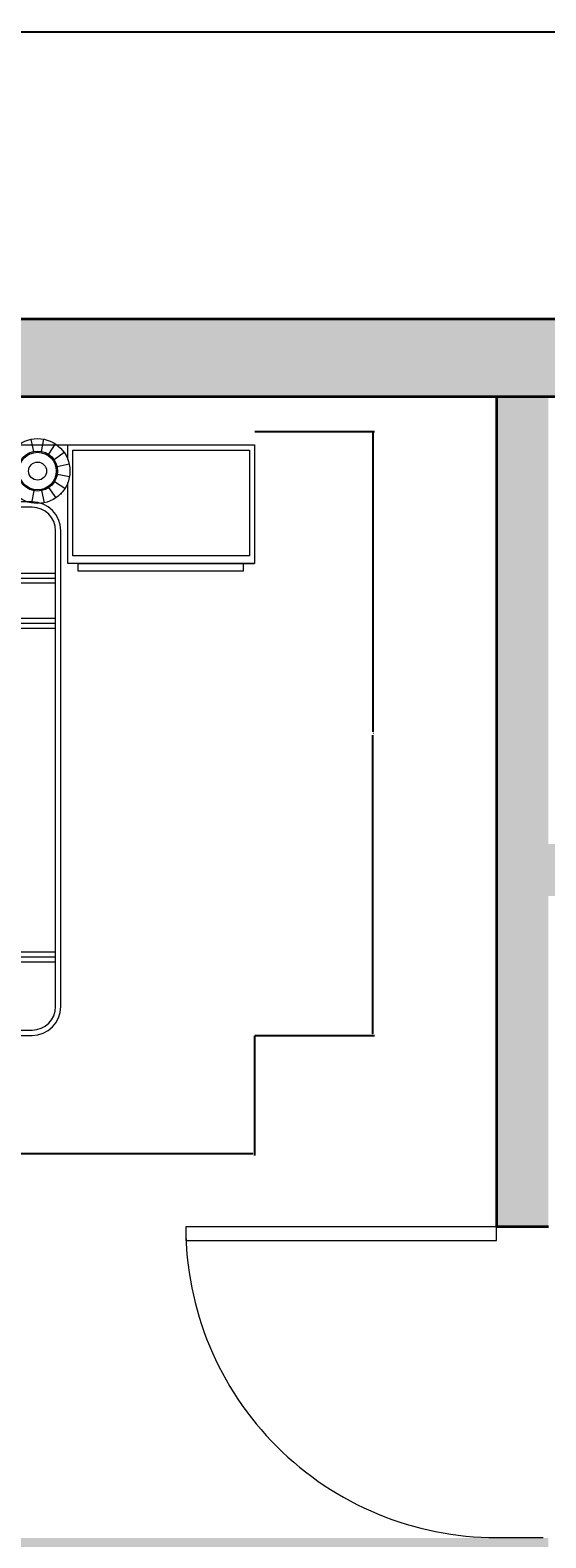
# Model space of a CAD drawing. Units: inches. Extents: x 2070 to 4408, y 1595 to 4269.
# Tile 14 of 20: x 2185 to 2245, y 2150 to 2325. Entities that reach past the tile are written whole.
import ezdxf

# ---------------------------------------------------------------- set-up
doc = ezdxf.new("R2010")
doc.units = ezdxf.units.IN
for name, color, linetype, lineweight in [('A-ANNO-DIMS', 2, 'Continuous', 18), ('A-DOOR', 4, 'Continuous', 18), ('A-FURN', 8, 'Continuous', 18), ('A-WALL', 7, 'Continuous', 35)]:
    doc.layers.add(name, color=color, linetype=linetype, lineweight=lineweight)
doc.layers.add('A-WALL-PATT', color=18, linetype='Continuous', lineweight=13, true_color=0x000000)
doc.styles.get("Standard").update_dxf_attribs({"font": 'arial.ttf'})
doc.dimstyles.get("Standard").update_dxf_attribs({"dimtxt": 0.18, "dimasz": 0.18, "dimexe": 0.18, "dimexo": 0.0625, "dimgap": 0.09, "dimtad": 0, "dimtih": 1, "dimtoh": 1, "dimdec": 4, "dimzin": 0, "dimdsep": 46, "dimtxsty": 'Standard', "dimcen": 0.09, "dimadec": 0, "dimazin": 0, "dimtfac": 1, "dimtdec": 4, "dimtofl": 0, "dimtmove": 0, "dimatfit": 3, "dimfxl": 1, "dimtolj": 1, "dimtzin": 0, "dimarcsym": 0})

# ---------------------------------------------------------------- blocks, each defined once
blk = doc.blocks.new('*U3')
for p, q in [((0, 0), (0, 6)), ((40, 0), (40, 6))]:
    blk.add_line(p, q)
blk.add_lwpolyline([(0, 0), (0, -40), (1.75, -40), (1.75, 0)], close=True)
blk.add_arc((0, 0), 40, 270, 0)
blk = doc.blocks.new('A$C18EB7ED0')
for p, q in [((0, 2.1539), (2.8801, 2.1539)), ((2.0643, 2.1733), (2.0739, 2.129)), ((2.1105, 2.1741), (2.1024, 2.1295)), ((2.1534, 2.1571), (2.1288, 2.119)), ((2.1997, 2.1), (2.1997, 2.1539)), ((2.8801, 2.1539), (2.8801, 1.7209)), ((2.1865, 2.1251), (2.1493, 2.0992)), ((2.2184, 2.1337), (2.8624, 2.1337)), ((2.2184, 1.7489), (2.2184, 2.1337)), ((2.8624, 2.1337), (2.8624, 1.7489)), ((2.2049, 2.0827), (2.1606, 2.0731)), ((2.2056, 2.0366), (2.161, 2.0447)), ((2.0682, 1.9414), (2.0763, 1.986)), ((2.1143, 1.9422), (2.1047, 1.9865)), ((2.1566, 1.9605), (2.1308, 1.9978)), ((2.1887, 1.9937), (2.1506, 2.0183)), ((2.1997, 1.7209), (2.1997, 2.0155)), ((2.0691, 1.9452), (0.8491, 1.9452)), ((2.0691, 1.926), (0.8491, 1.926)), ((2.1742, 1.9754), (2.1771, 1.9754)), ((2.1771, 1.9754), (2.1771, 1.9785)), ((2.155, 0.1052), (2.155, 1.8401)), ((2.1743, 0.1052), (2.1743, 1.8401)), ((2.8801, 1.7209), (2.1997, 1.7209)), ((2.8624, 1.7489), (2.2184, 1.7489)), ((2.2369, 1.7209), (2.8801, 1.7209)), ((2.2369, 1.6929), (2.2369, 1.7209)), ((2.839, 1.7209), (2.839, 1.6929)), ((1.9608, 1.6858), (2.155, 1.6858)), ((1.9608, 1.6678), (2.155, 1.6678)), ((1.9608, 1.6498), (2.155, 1.6498)), ((2.839, 1.6929), (2.2369, 1.6929)), ((0.7632, 1.5215), (2.155, 1.5215)), ((0.7632, 1.5035), (2.155, 1.5035)), ((0.7632, 1.4855), (2.155, 1.4855)), ((0.7632, 0.3045), (2.155, 0.3045)), ((0.7632, 0.2865), (2.155, 0.2865)), ((0.7632, 0.2685), (2.155, 0.2685)), ((0.8491, 0.0193), (2.0691, 0.0193)), ((0.8491, 0), (2.0691, 0))]:
    blk.add_line(p, q)
for radius in [0.1182, 0.0729, 0.0684, 0.0328]:
    blk.add_circle((2.0893, 2.0578), radius)
for centre, radius, start, end in [((2.0691, 1.8401), 0.1052, 0, 90), ((2.0691, 1.8401), 0.0859, 0, 90), ((2.0691, 0.1052), 0.1052, 270, 0), ((2.0691, 0.1052), 0.0859, 270, 0)]:
    blk.add_arc(centre, radius, start, end)
blk = doc.blocks.new('*D17')
at = {"layer": 'A-ANNO-DIMS', "color": 0, "lineweight": -2, "transparency": 16777216}
for p, q in [((2119.88, 2208.47), (2119.88, 2194.65)), ((2211.2, 2208.47), (2211.2, 2194.65)), ((2120.06, 2194.83), (2164.77, 2194.83)), ((2211.02, 2194.83), (2166.31, 2194.83))]:
    blk.add_line(p, q, dxfattribs=at)
at = {"layer": 'A-ANNO-DIMS', "color": 0, "transparency": 16777216}
for points in [[(2120.06, 2194.86), (2120.06, 2194.8), (2119.88, 2194.83)], [(2211.02, 2194.86), (2211.02, 2194.8), (2211.2, 2194.83)]]:
    blk.add_solid(points, dxfattribs=at)
at = {"layer": 'Defpoints', "color": 0, "transparency": 16777216}
for p in [(2119.88, 2208.53), (2211.2, 2208.53), (2211.2, 2194.83)]:
    blk.add_point(p, dxfattribs=at)
at = {"layer": 'A-ANNO-DIMS', "color": 0, "transparency": 16777216, "insert": (2165.54, 2194.83), "char_height": 0.18, "attachment_point": 5}
blk.add_mtext('\\A1;BED SET 91', dxfattribs=at)
blk = doc.blocks.new('*D18')
at = {"layer": 'A-ANNO-DIMS', "color": 0, "lineweight": -2, "transparency": 16777216}
for p, q in [((2211.26, 2278.36), (2225.08, 2278.36)), ((2224.9, 2278.18), (2224.9, 2243.63)), ((2224.9, 2208.71), (2224.9, 2243.26)), ((2211.26, 2208.53), (2225.08, 2208.53))]:
    blk.add_line(p, q, dxfattribs=at)
at = {"layer": 'A-ANNO-DIMS', "color": 0, "transparency": 16777216}
for points in [[(2224.87, 2278.18), (2224.93, 2278.18), (2224.9, 2278.36)], [(2224.87, 2208.71), (2224.93, 2208.71), (2224.9, 2208.53)]]:
    blk.add_solid(points, dxfattribs=at)
at = {"layer": 'Defpoints', "color": 0, "transparency": 16777216}
for p in [(2211.2, 2278.36), (2224.9, 2278.36), (2211.2, 2208.53)]:
    blk.add_point(p, dxfattribs=at)
at = {"layer": 'A-ANNO-DIMS', "color": 0, "transparency": 16777216, "insert": (2224.9, 2243.45), "char_height": 0.18, "attachment_point": 5}
blk.add_mtext('\\A1;70', dxfattribs=at)
blk = doc.blocks.new('*D23')
at = {"layer": 'A-ANNO-DIMS', "color": 0, "lineweight": -2, "transparency": 16777216}
for p, q in [((2103.2, 2291.46), (2103.2, 2324.76)), ((2103.38, 2324.58), (2278.91, 2324.58)), ((2455.02, 2324.58), (2279.48, 2324.58)), ((2455.2, 2291.46), (2455.2, 2324.76))]:
    blk.add_line(p, q, dxfattribs=at)
at = {"layer": 'A-ANNO-DIMS', "color": 0, "transparency": 16777216}
for points in [[(2103.38, 2324.61), (2103.38, 2324.55), (2103.2, 2324.58)], [(2455.02, 2324.61), (2455.02, 2324.55), (2455.2, 2324.58)]]:
    blk.add_solid(points, dxfattribs=at)
at = {"layer": 'Defpoints', "color": 0, "transparency": 16777216}
for p in [(2455.2, 2324.58), (2103.2, 2291.4), (2455.2, 2291.4)]:
    blk.add_point(p, dxfattribs=at)
at = {"layer": 'A-ANNO-DIMS', "color": 0, "transparency": 16777216, "insert": (2279.2, 2324.58), "char_height": 0.18, "attachment_point": 5}
blk.add_mtext('\\A1;352', dxfattribs=at)
blk = doc.blocks.new('*D24')
at = {"layer": 'A-ANNO-DIMS', "color": 0, "lineweight": -2, "transparency": 16777216}
for p, q in [((2103.13, 2291.4), (2069.84, 2291.4)), ((2070.02, 2291.22), (2070.02, 1960.08)), ((2070.02, 1628.58), (2070.02, 1959.72)), ((2336.13, 1628.4), (2069.84, 1628.4))]:
    blk.add_line(p, q, dxfattribs=at)
at = {"layer": 'A-ANNO-DIMS', "color": 0, "transparency": 16777216}
for points in [[(2069.99, 2291.22), (2070.05, 2291.22), (2070.02, 2291.4)], [(2069.99, 1628.58), (2070.05, 1628.58), (2070.02, 1628.4)]]:
    blk.add_solid(points, dxfattribs=at)
at = {"layer": 'Defpoints', "color": 0, "transparency": 16777216}
for p in [(2070.02, 2291.4), (2103.2, 2291.4), (2336.2, 1628.4)]:
    blk.add_point(p, dxfattribs=at)
at = {"layer": 'A-ANNO-DIMS', "color": 0, "transparency": 16777216, "insert": (2070.02, 1959.9), "char_height": 0.18, "attachment_point": 5}
blk.add_mtext('\\A1;663', dxfattribs=at)

msp = doc.modelspace()

# ---------------------------------------------------------------- hatches: boundary and pattern name
at = {"layer": 'A-WALL-PATT'}
h = msp.add_hatch(color=256, dxfattribs=at)
h.dxf.hatch_style = 1
h.paths.add_polyline_path([(2346.196, 2218.3995), (2346.196, 2282.3995), (2340.196, 2282.3995), (2340.196, 2212.3995), (2345.5866, 2212.3995), (2346.196, 2212.3995)], flags=0)
h.paths.add_polyline_path([(2245.196, 2282.3995), (2239.196, 2282.3995), (2239.196, 2186.3995), (2244.5866, 2186.3995), (2245.196, 2186.3995)], flags=0)
h.paths.add_polyline_path([(2340.196, 2230.6455), (2245.196, 2230.6455), (2245.196, 2224.6455), (2340.196, 2224.6455)], flags=0)
h.paths.add_polyline_path([(2245.196, 2150.3995), (2239.196, 2150.3995), (2164.4362, 2150.3995), (2164.4362, 2144.3995), (2239.196, 2144.3995), (2239.196, 2086.3995), (2239.196, 2067.2711), (2244.5866, 2067.2711), (2245.196, 2067.2711), (2245.196, 2144.3995)], flags=0)
h.paths.add_polyline_path([(2346.196, 2176.3995), (2340.196, 2176.3995), (2340.196, 2086.3995), (2346.196, 2086.3995), (2346.196, 2125.318)], flags=0)
h.paths.add_polyline_path([(2446.196, 2086.3995), (2346.196, 2086.3995), (2340.196, 2086.3995), (2340.196, 2080.3995), (2446.196, 2080.3995)], flags=0)
h.paths.add_polyline_path([(2455.196, 2291.3995), (2103.196, 2291.3995), (2103.196, 1699.3995), (2336.196, 1699.3995), (2336.196, 1628.3995), (2345.196, 1628.3995), (2446.196, 1628.3995), (2454.8846, 1628.3995), (2454.8846, 1699.3995)])
h.paths.add_polyline_path([(2446.196, 2282.3995), (2446.196, 2218.3995), (2446.196, 2212.3995), (2446.196, 2086.3995), (2446.196, 2080.3995), (2446.196, 1708.3995), (2446.196, 1637.3995), (2345.196, 1637.3995), (2345.196, 1699.3995), (2345.196, 1708.3995), (2336.196, 1708.3995), (2112.196, 1708.3995), (2112.196, 2282.3995), (2239.196, 2282.3995), (2245.196, 2282.3995), (2356.196, 2282.3995)], flags=16)
h.paths.add_polyline_path([(2245.196, 2150.3995), (2245.196, 2144.3995), (2245.196, 2067.2711), (2244.5866, 2067.2711), (2239.196, 2067.2711), (2239.196, 2065.6988), (2203.2929, 2065.6988, 0.40145271), (2239.196, 2031.3337), (2244.5866, 2031.3337), (2245.196, 2031.2711), (2245.196, 1924.1525), (2239.196, 1924.1525), (2239.196, 1922.5803), (2203.2929, 1922.5803, 0.40145271), (2239.196, 1888.2151), (2244.5866, 1888.2151), (2245.196, 1888.1525), (2245.196, 1748.3995), (2339.196, 1748.4621, -0.40145271), (2303.2929, 1782.8272), (2303.2585, 1782.8272), (2303.2585, 1784.3995), (2339.196, 1784.3995), (2339.196, 1877.2067), (2291.196, 1877.2067), (2291.196, 1883.2067), (2291.196, 1946.3995), (2291.196, 1952.3995), (2291.196, 2086.3995), (2297.196, 2086.3995), (2302.196, 2086.3995), (2302.196, 2081.0259), (2303.7633, 2081.0259), (2303.7633, 2080.3995), (2338.0148, 2080.3995, 0.00437129), (2338.0203, 2081.0259), (2338.0203, 2086.3995), (2340.196, 2086.3995), (2340.196, 2176.4621), (2345.5866, 2176.4621, 0.40145271), (2381.4896, 2210.8272), (2345.5866, 2210.8272), (2345.5866, 2212.3995), (2340.196, 2212.3995), (2340.196, 2224.6455), (2245.196, 2224.6455), (2245.196, 2186.3995), (2244.5866, 2186.3995), (2239.196, 2186.3995), (2239.196, 2184.8272), (2203.2929, 2184.8272, 0.40145271), (2239.196, 2150.4621), (2244.5866, 2150.4621)], flags=0)
h.paths.add_polyline_path([(2346.196, 2282.3995), (2346.196, 2218.3995), (2377.1813, 2218.3995), (2377.1813, 2212.3995), (2346.196, 2212.3995), (2345.5866, 2212.3995), (2340.196, 2212.3995), (2340.196, 2224.6455), (2245.196, 2224.6455), (2245.196, 2230.6455), (2245.196, 2282.3995), (2292.696, 2256.5225), (2340.196, 2282.3995)], flags=0)
h.paths.add_polyline_path([(2346.196, 2086.3995), (2340.196, 2086.3995), (2340.196, 2080.3995), (2446.196, 2080.3995), (2431.196, 2016.3995), (2446.196, 1952.3995), (2412.196, 1952.3995), (2412.196, 2080.3995), (2340.196, 2080.3995), (2340.196, 2086.3995), (2340.196, 2176.3995), (2346.196, 2176.3995), (2346.196, 2125.318)], flags=0)
h.paths.add_polyline_path([(2186.508, 2270.0471, -0.03755288), (2186.9712, 2269.8581), (2186.9164, 2270.112, -0.02759121)], flags=0)
h.paths.add_polyline_path([(2183.955, 2273.7766, 1), (2188.2945, 2273.7766, 1)], flags=0)
h.paths.add_polyline_path([(2142.5261, 2274.6158, -0.03707541), (2142.5672, 2275.1696), (2142.5672, 2276.826), (2119.8759, 2276.826), (2119.8759, 2263.0962), (2140.4332, 2263.0962), (2142.5672, 2263.0962), (2142.5672, 2274.0621, -0.03707541)], flags=0)
h.paths.add_polyline_path([(2209.8974, 2263.0962), (2209.8974, 2262.2079), (2190.8042, 2262.2079), (2190.8042, 2263.0962)], flags=0)
h.paths.add_polyline_path([(2210.6382, 2276.1833), (2210.6382, 2263.9844), (2190.2185, 2263.9844), (2190.2185, 2276.1833)], flags=0)
h.paths.add_polyline_path([(2188.4362, 2273.7766, -1), (2183.8133, 2273.7766, -1)], flags=0)
h.paths.add_polyline_path([(2245.196, 2150.3995), (2245.196, 2144.3995), (2245.196, 2067.2711), (2239.196, 2067.2711), (2239.196, 2080.3995), (2172.196, 2080.3995), (2172.196, 2000.3995), (2239.196, 2000.3995), (2239.196, 1940.3995), (2159.0187, 1940.3995), (2123.0187, 1940.3995), (2112.196, 1940.3995), (2112.196, 1946.3995), (2123.0187, 1946.3995), (2123.0187, 1982.2238), (2124.586, 1982.2238), (2124.586, 1982.1895, -0.40145271), (2158.8429, 1946.3995), (2159.0187, 1946.3995), (2239.196, 1946.3995), (2239.196, 1994.3995), (2112.196, 1994.3995), (2112.196, 2000.3995), (2139.196, 2040.3995), (2112.196, 2080.3995), (2112.196, 2086.3995), (2239.196, 2086.3995), (2239.196, 2144.3995), (2209.5809, 2144.3995), (2209.5809, 2136.3995), (2203.0809, 2136.3995), (2205.0809, 2130.3996, -0.70257121), (2199.081, 2116.3995, -0.70256205), (2193.0809, 2130.3994), (2195.0809, 2136.3995), (2192.0809, 2136.3995), (2192.0809, 2134.8995), (2189.0809, 2134.8995), (2189.0809, 2135.8995), (2191.0809, 2135.8995), (2191.0809, 2136.3995), (2188.5809, 2136.3995), (2188.5809, 2144.3995), (2164.2481, 2144.3995, -0.39385849), (2130.0035, 2109.5491), (2130.0035, 2109.5147), (2128.4362, 2109.5147), (2128.4362, 2144.3995), (2112.196, 2144.3995), (2112.196, 2150.3995), (2128.4362, 2150.3995), (2128.4362, 2150.7127), (2164.4362, 2150.7127), (2164.4362, 2150.3995), (2239.196, 2150.3995)], flags=0)
h.paths.add_polyline_path([(2188.2075, 2266.8735), (2188.2075, 2211.8632, -0.41421356), (2185.4833, 2209.1391), (2146.7995, 2209.1391, -0.41421356), (2144.0754, 2211.8632), (2144.0754, 2266.8735, -0.41421356), (2146.7995, 2269.5976), (2185.4833, 2269.5976, -0.41421356)], flags=0)
h.paths.add_polyline_path([(2185.0844, 2273.7766, -1), (2187.1651, 2273.7766, -1)], flags=0)
h.paths.add_polyline_path([(2182.0486, 2259.2932), (2168.0953, 2259.2932), (2168.0953, 2260.8424), (2163.7261, 2260.8424), (2163.7261, 2259.2932), (2149.7727, 2259.2932), (2149.7727, 2266.3352), (2163.7261, 2266.3352), (2163.7261, 2261.9839), (2168.0953, 2261.9839), (2168.0953, 2266.3352), (2182.0486, 2266.3352)], flags=0)
h.paths.add_polyline_path([(2148.2585, 2250.2051), (2153.0615, 2241.8861, 0.39807048)], flags=0)
h.paths.add_polyline_path([(2162.7572, 2247.2885), (2153.1461, 2241.7396), (2148.1083, 2250.4653), (2157.7194, 2256.0142)], flags=0)
h.paths.add_polyline_path([(2162.6726, 2247.4351, -0.39286196), (2157.8415, 2255.6313), (2157.6431, 2255.6313), (2157.8696, 2255.7541)], flags=0)
h.paths.add_polyline_path([(2164.2604, 2145.339), (2164.4362, 2144.3995), (2164.4362, 2150.3995), (2164.2604, 2150.7127)], flags=0)
h.paths.add_polyline_path([(2208.5809, 2142.6495), (2208.5809, 2138.3995, -0.41421356), (2207.8309, 2137.3995), (2190.5809, 2137.3995, -0.41421356), (2189.5809, 2138.1495), (2189.5809, 2142.3995, -0.41421356), (2190.3309, 2143.3995), (2207.5809, 2143.3995, -0.41421356)], flags=0)
h.paths.add_polyline_path([(2147.957, 2229.9119), (2154.7494, 2223.1195, 0.39807048)], flags=0)
h.paths.add_polyline_path([(2162.7165, 2230.8473), (2154.8691, 2222.9998), (2147.7446, 2230.1244), (2155.592, 2237.9718)], flags=0)
h.paths.add_polyline_path([(2162.5969, 2230.9669, -0.39807048), (2155.8044, 2237.7594)], flags=0)
h.paths.add_polyline_path([(2391.8776, 2049.9192), (2408.5766, 2049.9192), (2408.5766, 2033.2202), (2408.5766, 1983.123), (2408.5766, 1966.4239), (2391.8776, 1966.4239), (2391.8776, 1983.123), (2341.7804, 1983.123), (2341.7804, 2033.2202), (2391.8776, 2033.2202)], flags=0)
h.paths.add_polyline_path([(2144.1055, 2274.6158, 1), (2148.445, 2274.6158, 1)], flags=0)
h.paths.add_polyline_path([(2148.5867, 2274.6158, -1), (2143.9638, 2274.6158, -1)], flags=0)
h.paths.add_polyline_path([(2145.2349, 2274.6158, -1), (2147.3156, 2274.6158, -1)], flags=0)
edge = h.paths.add_edge_path(flags=0)
edge.add_ellipse((2400.5951, 2040.9436), major_axis=(-4.5109, 0), ratio=0.97544784, start_angle=180, end_angle=270, ccw=False)
edge.add_ellipse((2400.5951, 2040.9436), major_axis=(-4.5109, 0), ratio=0.97544784, start_angle=90, end_angle=180, ccw=False)
edge.add_ellipse((2400.5951, 2040.9436), major_axis=(-4.5109, 0), ratio=0.97544784, start_angle=0, end_angle=90, ccw=False)
edge.add_ellipse((2400.5951, 2040.9436), major_axis=(-4.5109, 0), ratio=0.97544784, start_angle=270, end_angle=360, ccw=False)
h.paths.add_polyline_path([(2199.0809, 2117.3995, -0.73452973), (2195.0809, 2130.3995), (2203.081, 2130.3995, -0.73453329)], flags=0)
h.paths.add_polyline_path([(2141.9147, 2276.0353), (2141.9147, 2263.9844), (2120.4685, 2263.9844), (2120.4685, 2276.0353)], flags=0)
h.paths.add_polyline_path([(2138.4481, 2273.4072), (2138.4481, 2266.7226), (2133.2801, 2266.7226), (2133.2801, 2273.4072)], flags=0)
h.paths.add_polyline_path([(2137.9691, 2272.9175), (2137.9691, 2272.204), (2135.4229, 2272.204), (2135.4229, 2271.6329), (2135.3221, 2270.1051), (2135.3221, 2269.0265), (2135.4229, 2268.6811), (2135.4229, 2267.2011), (2133.7212, 2267.2011), (2133.7212, 2268.6811), (2133.7983, 2269.9587), (2133.7983, 2271.2758), (2133.7212, 2271.6329), (2133.7212, 2273.0065), (2135.717, 2273.0065), (2135.717, 2272.9175)], flags=0)
h.paths.add_polyline_path([(2137.9215, 2271.8264), (2137.9215, 2271.3786), (2137.5182, 2271.3786), (2136.9355, 2271.3786), (2136.3529, 2271.3786), (2135.7703, 2271.3786), (2135.7703, 2271.8264), (2136.1736, 2271.8264), (2136.7562, 2271.8264), (2137.3389, 2271.8264)], flags=0)
h.paths.add_polyline_path([(2137.9215, 2271.692), (2137.5182, 2271.692), (2136.9355, 2271.513), (2137.3389, 2271.513)], flags=0)
h.paths.add_polyline_path([(2136.3529, 2271.692), (2135.7703, 2271.513), (2136.1736, 2271.513), (2136.7562, 2271.692)], flags=0)
h.paths.add_polyline_path([(2137.9215, 2271.513), (2137.5182, 2271.513), (2136.7562, 2271.747), (2136.7562, 2271.692), (2137.3389, 2271.692)], flags=0)
h.paths.add_polyline_path([(2137.8207, 2270.4664), (2137.8207, 2270.0971), (2137.8207, 2269.627), (2137.8207, 2269.1569), (2137.8207, 2268.6868), (2137.3837, 2268.6868), (2136.6442, 2268.6868), (2135.9271, 2268.6868), (2135.9271, 2269.0562), (2135.9271, 2269.5263), (2135.9271, 2269.9963), (2135.9271, 2270.4664), (2136.3641, 2270.4664), (2137.0812, 2270.4664)], flags=0)
h.paths.add_polyline_path([(2137.3837, 2269.627), (2137.8207, 2269.627), (2137.8207, 2269.5263), (2137.3837, 2269.5263), (2137.3837, 2269.1569), (2137.8207, 2269.1569), (2137.3837, 2269.0562), (2137.3837, 2268.6868), (2137.0812, 2268.6868), (2137.0812, 2269.0562), (2136.6442, 2269.0562), (2136.6442, 2268.6868), (2136.3641, 2268.6868), (2136.3641, 2269.0562), (2135.9271, 2269.0562), (2135.9271, 2269.1569), (2136.3641, 2269.1569), (2136.3641, 2269.5263), (2135.9271, 2269.5263), (2135.9271, 2269.627), (2136.3641, 2269.627), (2136.3641, 2269.9963), (2135.9271, 2269.9963), (2136.3641, 2270.0971), (2136.3641, 2270.4664), (2136.6442, 2270.4664), (2136.6442, 2270.0971), (2137.0812, 2270.0971), (2137.0812, 2270.4664), (2137.3837, 2270.4664), (2137.3837, 2270.0971), (2137.8207, 2270.0971), (2137.3837, 2269.9963)], flags=0)
h.paths.add_polyline_path([(2137.5182, 2271.8264), (2137.5182, 2271.692), (2137.3389, 2271.3786), (2137.3389, 2271.513)], flags=0)
h.paths.add_polyline_path([(2137.8179, 2267.8138), (2137.8179, 2267.6879), (2137.1876, 2267.6879), (2136.4733, 2267.6879), (2135.759, 2267.6879), (2135.759, 2267.8138), (2136.3893, 2267.8138), (2137.1036, 2267.8138)], flags=0)
h.paths.add_polyline_path([(2137.0812, 2269.9963), (2137.0812, 2269.627), (2137.0812, 2269.1569), (2136.6442, 2269.1569), (2136.6442, 2269.5263), (2136.6442, 2269.9963)], flags=0)
h.paths.add_polyline_path([(2136.3529, 2271.8264), (2136.3529, 2271.692), (2136.1736, 2271.3786), (2136.1736, 2271.513)], flags=0)
h.paths.add_polyline_path([(2136.4733, 2267.8138), (2136.4733, 2267.6879), (2136.3893, 2267.6879), (2136.3893, 2267.8138)], flags=0)
h.paths.add_polyline_path([(2407.9087, 2032.5522), (2407.9087, 1983.7909), (2359.81, 1983.7909, -0.00912788), (2359.0575, 1983.7909), (2342.4483, 1983.7909), (2342.4483, 2032.5522)], flags=0)
h.paths.add_polyline_path([(2389.1838, 2023.1358), (2353.7856, 2023.1358), (2353.7856, 1985.4867, -0.09210376), (2350.2788, 1988.655), (2350.2788, 2026.6426), (2389.1838, 2026.6426)], flags=0)
h.paths.add_polyline_path([(2352.6166, 2024.3048), (2351.4477, 2024.3048), (2351.4477, 2025.4737), (2352.6166, 2025.4737)], flags=0)
h.paths.add_polyline_path([(2399.6319, 2026.7589), (2404.3661, 2026.7589, -0.41421356), (2407.0379, 2024.087), (2407.0379, 2013.4908, -0.41421356), (2404.3661, 2010.819), (2399.6319, 2010.819, -0.41421356), (2396.96, 2013.4908), (2396.96, 2024.087, -0.41421356)], flags=0)
h.paths.add_polyline_path([(2399.6319, 2026.0909), (2404.3661, 2026.0909, -0.41421356), (2406.37, 2024.087), (2406.37, 2013.4908, -0.41421356), (2404.3661, 2011.487), (2399.6319, 2011.487, -0.41421356), (2397.628, 2013.4908), (2397.628, 2024.087, -0.41421356)], flags=0)
h.paths.add_polyline_path([(2399.6319, 2002.3217), (2404.3661, 2002.3217, -0.41421356), (2407.0379, 1999.6498), (2407.0379, 1989.0536, -0.41421356), (2404.3661, 1986.3818), (2399.6319, 1986.3818, -0.41421356), (2396.96, 1989.0536), (2396.96, 1999.6498, -0.41421356)], flags=0)
h.paths.add_polyline_path([(2399.6319, 2001.6537), (2404.3661, 2001.6537, -0.41421356), (2406.37, 1999.6498), (2406.37, 1989.0536, -0.41421356), (2404.3661, 1987.0497), (2399.6319, 1987.0497, -0.41421356), (2397.628, 1989.0536), (2397.628, 1999.6498, -0.41421356)], flags=0)
edge = h.paths.add_edge_path(flags=0)
edge.add_ellipse((2400.5951, 1975.3996), major_axis=(-4.5109, 0), ratio=0.97544784, start_angle=-180, end_angle=-90, ccw=False)
edge.add_ellipse((2400.5951, 1975.3996), major_axis=(-4.5109, 0), ratio=0.97544784, start_angle=90, end_angle=180, ccw=False)
edge.add_ellipse((2400.5951, 1975.3996), major_axis=(-4.5109, 0), ratio=0.97544784, start_angle=0, end_angle=90, ccw=False)
edge.add_ellipse((2400.5951, 1975.3996), major_axis=(-4.5109, 0), ratio=0.97544784, start_angle=-90, end_angle=0, ccw=False)
h.paths.add_polyline_path([(2345.196, 1910.3995), (2366.4386, 1910.3995), (2366.4386, 1925.4555), (2392.3856, 1925.4555), (2392.3856, 1933.5025), (2400.1399, 1925.4555), (2392.3856, 1919.8795), (2392.3856, 1925.4555), (2366.4386, 1925.4555), (2366.4386, 1910.3995), (2381.196, 1910.3995), (2405.196, 1910.3995), (2405.196, 1898.3995), (2446.196, 1898.3995), (2446.196, 1886.3995), (2405.196, 1886.3995), (2405.196, 1874.3995), (2446.196, 1874.3995), (2446.196, 1862.3995), (2405.196, 1862.3995), (2405.196, 1850.3995), (2446.196, 1850.3995), (2446.196, 1838.3995), (2405.196, 1838.3995), (2405.196, 1826.3995), (2446.196, 1826.3995), (2446.196, 1814.3995), (2405.196, 1814.3995), (2405.196, 1802.3995), (2446.196, 1802.3995), (2446.196, 1798.3995), (2446.196, 1792.3995), (2405.196, 1792.3995), (2405.196, 1910.3995), (2381.196, 1910.3995), (2381.196, 1792.3995), (2345.196, 1792.3995)], flags=0)
h.paths.add_polyline_path([(2333.0944, 1863.3993, -0.41421356), (2334.7225, 1861.7712), (2334.7225, 1859.329), (2335.2653, 1859.329, -0.41421356), (2337.4361, 1857.1582), (2337.4361, 1843.862, -0.41421356), (2335.2653, 1841.6911, -0.41421356), (2337.4361, 1839.5203), (2337.4361, 1827.5808, -0.41421356), (2335.2653, 1825.41, -0.41421356), (2337.4361, 1823.2392), (2337.4361, 1808.5862, -0.41421356), (2335.2653, 1806.4153), (2334.7225, 1806.4153), (2334.7225, 1803.9732, -0.41421356), (2333.0944, 1802.3451), (2317.356, 1802.3451), (2317.0846, 1802.3451, -0.41421356), (2315.7279, 1803.7018), (2315.7279, 1803.8646), (2313.8284, 1803.8646, -0.41421356), (2311.6576, 1806.0354), (2311.6576, 1823.2015, -0.39597602), (2313.6834, 1825.3765, -0.43384798), (2311.6576, 1827.2718), (2311.6576, 1839.761, -0.41421356), (2313.5571, 1841.6604), (2313.8284, 1841.6604), (2333.8159, 1841.6604, -0.04213623), (2334.1798, 1841.6911, -0.41421356), (2332.009, 1843.862), (2332.009, 1857.1582, -0.41421356), (2334.1798, 1859.329), (2317.356, 1859.329), (2317.0846, 1859.329, -0.41421356), (2315.7279, 1860.6858), (2315.7279, 1862.0426, -0.41421356), (2317.0846, 1863.3993), (2317.356, 1863.3993)], flags=0)
h.paths.add_polyline_path([(2208.8475, 1848.9818), (2208.8475, 1840.9741, -0.41421356), (2207.0458, 1839.1724), (2206.5453, 1839.1721), (2206.5453, 1838.7218, -0.40985861), (2204.7704, 1836.9203), (2183.7501, 1836.9203, -0.41858196), (2181.9216, 1838.7218), (2181.9216, 1839.1721), (2181.421, 1839.1724, -0.41421356), (2179.6193, 1840.9741), (2179.6193, 1848.6817, -0.44064415), (2185.1126, 1854.9874), (2203.3852, 1854.9874, -0.45707961)], flags=0)
h.paths.add_polyline_path([(2204.243, 1848.4815), (2204.243, 1848.4815, 0.41725335), (2202.2204, 1850.4833), (2186.2049, 1850.4833, 0.4111805), (2184.2237, 1848.4815), (2184.2237, 1848.4815, -0.4111807), (2186.2049, 1850.4833), (2202.2204, 1850.4833, -0.41725315)], flags=0)
h.paths.add_polyline_path([(2234.7177, 1830.228), (2234.7176, 1781.6047, -0.41421356), (2233.4381, 1780.3252), (2218.6064, 1780.3252, -0.41421356), (2217.8387, 1781.0929), (2217.8387, 1783.3961, -0.41421356), (2218.6064, 1784.1639), (2218.6065, 1796.9595, -0.41421356), (2219.886, 1798.239, -0.41421356), (2218.6065, 1799.5186), (2218.6065, 1812.3142, -0.41421356), (2219.8861, 1813.5938, -0.41421356), (2218.6065, 1814.8733), (2218.6065, 1827.6689, -0.41421356), (2217.8388, 1828.4367), (2217.8388, 1830.7399, -0.41421356), (2218.6065, 1831.5076), (2233.4382, 1831.5076, -0.41421356)], flags=0)
h.paths.add_polyline_path([(2230.6344, 1827.6689, -0.41421356), (2231.4021, 1826.9012), (2231.4021, 1784.9316, -0.41421356), (2230.6343, 1784.1639), (2221.1853, 1784.1639), (2221.1853, 1827.6689)], flags=0)
h.paths.add_polyline_path([(2222.7208, 1798.239), (2221.6971, 1798.239), (2221.6971, 1813.5938), (2222.7208, 1813.5938)], flags=0)
h.paths.add_polyline_path([(2206.5453, 1773.935), (2206.5453, 1773.4848), (2206.9457, 1773.4848), (2207.0458, 1773.4845, -0.41421356), (2208.8475, 1771.6827), (2208.8475, 1763.675, -0.44222432), (2203.6505, 1757.6695), (2185.3851, 1757.6695, -0.45508402), (2179.6193, 1763.9752), (2179.6193, 1771.6827, -0.41421356), (2181.421, 1773.4845), (2181.421, 1773.4848), (2181.9216, 1773.4848), (2181.9216, 1773.935, -0.40985861), (2183.6965, 1775.7366), (2204.7167, 1775.7366, -0.41858196)], flags=0)
h.paths.add_polyline_path([(2202.2619, 1762.1736), (2186.2464, 1762.1736, -0.41725315), (2184.2237, 1764.1754), (2184.2237, 1764.1754, 0.41725335), (2186.2464, 1762.1736), (2202.2619, 1762.1736, 0.4111805), (2204.243, 1764.1754), (2204.243, 1764.1754, -0.4111807)], flags=0)
h.paths.add_polyline_path([(2313.0034, 1713.1906), (2312.997, 1713.1697), (2313.0123, 1713.1612)], flags=0)
h.paths.add_polyline_path([(2305.7314, 1721.0488), (2305.6257, 1721.1994), (2305.4853, 1721.084)], flags=0)
h.paths.add_polyline_path([(2307.5562, 1726.1427), (2307.6186, 1726.1026), (2307.5737, 1726.0477), (2308.5692, 1720.6434), (2310.5345, 1721.2985), (2310.5721, 1721.411), (2310.6958, 1721.3523), (2313.8453, 1722.4021), (2314.9351, 1723.8033), (2314.9294, 1723.9165), (2315.0028, 1723.8903), (2313.874, 1722.4389), (2313.8697, 1722.4102), (2308.5692, 1720.6434), (2308.9864, 1720.122), (2309.0665, 1720.0971), (2309.053, 1720.0387), (2310.9235, 1717.7005), (2311.4182, 1717.6259), (2311.2918, 1717.2402), (2312.0655, 1716.2731), (2312.1081, 1716.2606), (2312.0969, 1716.2339), (2308.5692, 1720.6434), (2305.2249, 1717.745), (2305.232, 1717.704), (2305.1665, 1717.6944), (2308.5692, 1720.6434)], flags=0)
h.paths.add_polyline_path([(2288.2072, 1714.3431), (2288.2008, 1714.3222), (2288.216, 1714.3137)], flags=0)
h.paths.add_polyline_path([(2280.9352, 1722.2013), (2280.8295, 1722.3519), (2280.689, 1722.2365)], flags=0)
h.paths.add_polyline_path([(2282.76, 1727.2952), (2282.8224, 1727.2551), (2282.7775, 1727.2002), (2283.773, 1721.7959), (2285.7383, 1722.451), (2285.7759, 1722.5635), (2285.8995, 1722.5048), (2289.0491, 1723.5546), (2290.1389, 1724.9558), (2290.1332, 1725.069), (2290.2065, 1725.0428), (2289.0777, 1723.5915), (2289.0735, 1723.5628), (2283.773, 1721.7959), (2284.1901, 1721.2745), (2284.2703, 1721.2496), (2284.2567, 1721.1913), (2286.1273, 1718.8531), (2286.622, 1718.7785), (2286.4956, 1718.3927), (2287.2692, 1717.4256), (2287.3119, 1717.4131), (2287.3006, 1717.3864), (2283.773, 1721.7959), (2280.4286, 1718.8975), (2280.4357, 1718.8565), (2280.3703, 1718.8469), (2283.773, 1721.7959)], flags=0)
h.paths.add_polyline_path([(2302.0672, 1721.8694), (2301.8205, 1721.8572), (2301.7578, 1722.1787), (2299.415, 1724.5215), (2299.103, 1724.4694), (2299.0662, 1724.8703)], flags=0)
h.paths.add_polyline_path([(2264.5643, 1715.4956), (2264.5579, 1715.4747), (2264.5731, 1715.4662)], flags=0)
h.paths.add_polyline_path([(2257.2923, 1723.3538), (2257.1865, 1723.5044), (2257.0461, 1723.389)], flags=0)
h.paths.add_polyline_path([(2259.117, 1728.4477), (2259.1795, 1728.4077), (2259.1345, 1728.3527), (2260.13, 1722.9484), (2262.0954, 1723.6036), (2262.133, 1723.716), (2262.2566, 1723.6573), (2265.4061, 1724.7071), (2266.4959, 1726.1083), (2266.4902, 1726.2215), (2266.5636, 1726.1953), (2265.4348, 1724.744), (2265.4305, 1724.7153), (2260.13, 1722.9484), (2260.5472, 1722.427), (2260.6273, 1722.4022), (2260.6138, 1722.3438), (2262.4843, 1720.0056), (2262.979, 1719.931), (2262.8526, 1719.5452), (2263.6263, 1718.5781), (2263.6689, 1718.5656), (2263.6577, 1718.5389), (2260.13, 1722.9484), (2256.7857, 1720.05), (2256.7928, 1720.009), (2256.7273, 1719.9994), (2260.13, 1722.9484)], flags=0)
h.paths.add_polyline_path([(2277.2709, 1723.0219), (2277.0243, 1723.0097), (2276.9616, 1723.3312), (2274.6187, 1725.6741), (2274.3067, 1725.6219), (2274.27, 1726.0228)], flags=0)
h.paths.add_polyline_path([(2253.628, 1724.1744), (2253.3814, 1724.1622), (2253.3186, 1724.4838), (2250.9758, 1726.8266), (2250.6638, 1726.7744), (2250.627, 1727.1753)], flags=0)
h.paths.add_polyline_path([(2161.9194, 1715.4956), (2161.913, 1715.4747), (2161.9282, 1715.4662)], flags=0)
h.paths.add_polyline_path([(2154.6474, 1723.3538), (2154.5416, 1723.5044), (2154.4012, 1723.389)], flags=0)
h.paths.add_polyline_path([(2162.7899, 1724.744), (2162.7856, 1724.7153), (2157.4851, 1722.9484), (2157.9023, 1722.427), (2157.9824, 1722.4022), (2157.9689, 1722.3438), (2159.8394, 1720.0056), (2160.3341, 1719.931), (2160.2078, 1719.5452), (2160.9814, 1718.5781), (2161.024, 1718.5656), (2161.0128, 1718.5389), (2157.4851, 1722.9484), (2154.1408, 1720.05), (2154.1479, 1720.009), (2154.0824, 1719.9994), (2157.4851, 1722.9484), (2156.4721, 1728.4477), (2156.5346, 1728.4077), (2156.4896, 1728.3527), (2157.4851, 1722.9484), (2159.4505, 1723.6036), (2159.4881, 1723.716), (2159.6117, 1723.6573), (2162.7612, 1724.7071), (2163.851, 1726.1083), (2163.8453, 1726.2215), (2163.9187, 1726.1953)], flags=0)
h.paths.add_polyline_path([(2150.9831, 1724.1744), (2150.7365, 1724.1622), (2150.6738, 1724.4838), (2148.3309, 1726.8266), (2148.0189, 1726.7744), (2147.9822, 1727.1753)], flags=0)
h.paths.add_polyline_path([(2132.5099, 1716.6482), (2132.5035, 1716.6272), (2132.5187, 1716.6187)], flags=0)
h.paths.add_polyline_path([(2125.2379, 1724.5064), (2125.1322, 1724.6569), (2124.9917, 1724.5415)], flags=0)
h.paths.add_polyline_path([(2133.3804, 1725.8965), (2133.3762, 1725.8678), (2128.0757, 1724.101), (2128.4928, 1723.5795), (2128.5729, 1723.5547), (2128.5594, 1723.4963), (2130.43, 1721.1581), (2130.9246, 1721.0835), (2130.7983, 1720.6977), (2131.5719, 1719.7306), (2131.6146, 1719.7181), (2131.6033, 1719.6914), (2128.0757, 1724.101), (2124.7313, 1721.2025), (2124.7384, 1721.1615), (2124.6729, 1721.1519), (2128.0757, 1724.101), (2127.0626, 1729.6002), (2127.1251, 1729.5602), (2127.0801, 1729.5052), (2128.0757, 1724.101), (2130.041, 1724.7561), (2130.0786, 1724.8685), (2130.2022, 1724.8098), (2133.3517, 1725.8597), (2134.4415, 1727.2608), (2134.4358, 1727.3741), (2134.5092, 1727.3478)], flags=0)
h.paths.add_polyline_path([(2121.5736, 1725.3269), (2121.327, 1725.3148), (2121.2643, 1725.6363), (2118.9214, 1727.9791), (2118.6094, 1727.9269), (2118.5727, 1728.3279)], flags=0)
h.paths.add_polyline_path([(2433.3904, 1646.406), (2433.384, 1646.3851), (2433.3992, 1646.3766)], flags=0)
h.paths.add_polyline_path([(2426.1184, 1654.2642), (2426.0127, 1654.4148), (2425.8722, 1654.2994)], flags=0)
h.paths.add_polyline_path([(2427.9432, 1659.3581), (2428.0056, 1659.318), (2427.9606, 1659.2631), (2428.9562, 1653.8588), (2430.9215, 1654.514), (2430.9591, 1654.6264), (2431.0827, 1654.5677), (2434.2323, 1655.6175), (2435.322, 1657.0187), (2435.3163, 1657.1319), (2435.3897, 1657.1057), (2434.2609, 1655.6544), (2434.2567, 1655.6257), (2428.9562, 1653.8588), (2429.3733, 1653.3374), (2429.4534, 1653.3126), (2429.4399, 1653.2542), (2431.3105, 1650.916), (2431.8051, 1650.8414), (2431.6788, 1650.4556), (2432.4524, 1649.4885), (2432.4951, 1649.476), (2432.4838, 1649.4493), (2428.9562, 1653.8588), (2425.6118, 1650.9604), (2425.6189, 1650.9194), (2425.5535, 1650.9098), (2428.9562, 1653.8588)], flags=0)
h.paths.add_polyline_path([(2376.63, 1645.4912), (2376.6236, 1645.4703), (2376.6388, 1645.4617)], flags=0)
h.paths.add_polyline_path([(2369.358, 1653.3494), (2369.2523, 1653.5), (2369.1118, 1653.3845)], flags=0)
h.paths.add_polyline_path([(2371.1828, 1658.4432), (2371.2452, 1658.4032), (2371.2003, 1658.3482), (2372.1958, 1652.944), (2374.1611, 1653.5991), (2374.1987, 1653.7116), (2374.3224, 1653.6528), (2377.4719, 1654.7027), (2378.5617, 1656.1038), (2378.556, 1656.2171), (2378.6293, 1656.1908), (2377.5005, 1654.7395), (2377.4963, 1654.7108), (2372.1958, 1652.944), (2372.6129, 1652.4225), (2372.6931, 1652.3977), (2372.6795, 1652.3393), (2374.5501, 1650.0011), (2375.0448, 1649.9265), (2374.9184, 1649.5407), (2375.692, 1648.5737), (2375.7347, 1648.5611), (2375.7234, 1648.5344), (2372.1958, 1652.944), (2368.8514, 1650.0456), (2368.8586, 1650.0046), (2368.7931, 1649.995), (2372.1958, 1652.944)], flags=0)
h.paths.add_polyline_path([(2404.0947, 1645.0338), (2404.0883, 1645.0128), (2404.1035, 1645.0043)], flags=0)
h.paths.add_polyline_path([(2396.8227, 1652.892), (2396.717, 1653.0425), (2396.5765, 1652.9271)], flags=0)
h.paths.add_polyline_path([(2398.6475, 1657.9858), (2398.7099, 1657.9458), (2398.665, 1657.8908), (2399.6605, 1652.4866), (2401.6258, 1653.1417), (2401.6634, 1653.2541), (2401.7871, 1653.1954), (2404.9366, 1654.2453), (2406.0264, 1655.6464), (2406.0207, 1655.7596), (2406.094, 1655.7334), (2404.9652, 1654.2821), (2404.961, 1654.2534), (2399.6605, 1652.4866), (2400.0776, 1651.9651), (2400.1578, 1651.9403), (2400.1442, 1651.8819), (2402.0148, 1649.5437), (2402.5095, 1649.4691), (2402.3831, 1649.0833), (2403.1567, 1648.1162), (2403.1994, 1648.1037), (2403.1881, 1648.077), (2399.6605, 1652.4866), (2396.3162, 1649.5881), (2396.3233, 1649.5471), (2396.2578, 1649.5375), (2399.6605, 1652.4866)], flags=0)
h.paths.add_polyline_path([(2419.4532, 1658.0857), (2422.4541, 1655.0848), (2422.2075, 1655.0726), (2422.1448, 1655.3941), (2419.8019, 1657.737), (2419.4899, 1657.6848)], flags=0)
h.paths.add_polyline_path([(2390.1575, 1656.7135), (2393.1584, 1653.7125), (2392.9118, 1653.7004), (2392.8491, 1654.0219), (2390.5063, 1656.3647), (2390.1943, 1656.3125)], flags=0)
h.paths.add_polyline_path([(2362.6928, 1657.1709), (2365.6937, 1654.1699), (2365.4471, 1654.1578), (2365.3844, 1654.4793), (2363.0416, 1656.8221), (2362.7295, 1656.77)], flags=0)
h.paths.add_polyline_path([(2419.9523, 2037.8601), (2440.2872, 2037.8601), (2440.2872, 2047.1732), (2419.9523, 2047.1732)], flags=8)
h.paths.add_polyline_path([(2370.186, 1698.9005), (2413.6287, 1698.9005), (2413.6287, 1708.0908), (2370.186, 1708.0908)], flags=8)
h.paths.add_polyline_path([(2370.1656, 1708.5185), (2430.0857, 1708.5185), (2430.0857, 1717.8316), (2370.1656, 1717.8316)], flags=8)
h.paths.add_polyline_path([(2254.1469, 1788.1883), (2302.2471, 1788.1883), (2302.2471, 1797.3786), (2254.1469, 1797.3786)], flags=8)
h.paths.add_polyline_path([(2254.1264, 1797.8063), (2326.1448, 1797.8063), (2326.1448, 1807.1194), (2254.1264, 1807.1194)], flags=8)
h.paths.add_polyline_path([(2300.08, 1914.5069), (2338.861, 1914.5069), (2338.861, 1923.6972), (2300.08, 1923.6972)], flags=8)
h.paths.add_polyline_path([(2300.0595, 1924.1249), (2331.5882, 1924.1249), (2331.5882, 1933.438), (2300.0595, 1933.438)], flags=8)
h.paths.add_polyline_path([(2176.6905, 1716.4567), (2224.1441, 1716.4567), (2224.1441, 1725.647), (2176.6905, 1725.647)], flags=8)
h.paths.add_polyline_path([(2176.67, 1726.0747), (2245.9176, 1726.0747), (2245.9176, 1735.3878), (2176.67, 1735.3878)], flags=8)
h.paths.add_polyline_path([(2339.997, 2039.7696), (2388.1034, 2039.7696), (2388.1034, 2048.9661), (2339.997, 2048.9661)], flags=8)
h.paths.add_polyline_path([(2339.9776, 2049.3928), (2388.7204, 2049.3928), (2388.7204, 2058.7059), (2339.9776, 2058.7059)], flags=8)
h.paths.add_polyline_path([(2366.0063, 2161.3825), (2409.449, 2161.3825), (2409.449, 2170.5728), (2366.0063, 2170.5728)], flags=8)
h.paths.add_polyline_path([(2365.9868, 2171.0016), (2405.879, 2171.0016), (2405.879, 2180.3085), (2365.9868, 2180.3085)], flags=8)
h.paths.add_polyline_path([(2366.0102, 2247.0726), (2407.12, 2247.0726), (2407.12, 2256.263), (2366.0102, 2256.263)], flags=8)
h.paths.add_polyline_path([(2365.9897, 2256.6906), (2397.9686, 2256.6906), (2397.9686, 2266.0037), (2365.9897, 2266.0037)], flags=8)
h.paths.add_polyline_path([(2271.8465, 2102.7885), (2307.6541, 2102.7885), (2307.6541, 2111.9849), (2271.8465, 2111.9849)], flags=8)
h.paths.add_polyline_path([(2271.8281, 2112.4126), (2304.2673, 2112.4126), (2304.2673, 2121.7196), (2271.8281, 2121.7196)], flags=8)
h.paths.add_polyline_path([(2141.6408, 2187.5934), (2182.108, 2187.5934), (2182.108, 2196.7837), (2141.6408, 2196.7837)], flags=8)
h.paths.add_polyline_path([(2141.6203, 2197.2114), (2190.3631, 2197.2114), (2190.3631, 2206.5245), (2141.6203, 2206.5245)], flags=8)
h.paths.add_polyline_path([(2165.7271, 2103.039), (2211.5027, 2103.039), (2211.5027, 2112.2293), (2165.7271, 2112.2293)], flags=8)
h.paths.add_polyline_path([(2165.7077, 2112.658), (2185.1033, 2112.658), (2185.1033, 2121.965), (2165.7077, 2121.965)], flags=8)
h.paths.add_polyline_path([(2174.945, 2048.0789), (2211.3973, 2048.0789), (2211.3973, 2057.2693), (2174.945, 2057.2693)], flags=8)
h.paths.add_polyline_path([(2174.9256, 2057.698), (2194.3212, 2057.698), (2194.3212, 2067.0049), (2174.9256, 2067.0049)], flags=8)
h.paths.add_polyline_path([(2164.8305, 1965.8394), (2202.9649, 1965.8394), (2202.9649, 1975.0297), (2164.8305, 1975.0297)], flags=8)
h.paths.add_polyline_path([(2164.8111, 1975.4584), (2184.2067, 1975.4584), (2184.2067, 1984.7654), (2164.8111, 1984.7654)], flags=8)
h.paths.add_polyline_path([(2133.0392, 1862.086), (2173.5065, 1862.086), (2173.5065, 1871.2763), (2133.0392, 1871.2763)], flags=8)
h.paths.add_polyline_path([(2133.0709, 1871.8585), (2157.0382, 1871.8585), (2157.0382, 1880.8585), (2133.0709, 1880.8585)], flags=8)
h.paths.add_polyline_path([(2406.4423, 1923.5541), (2418.8209, 1923.5541), (2418.8209, 1932.7199), (2406.4423, 1932.7199)], flags=8)
h = msp.add_hatch(color=256, dxfattribs=at)
h.dxf.hatch_style = 1
h.paths.add_polyline_path([(2245.196, 2282.3995), (2239.196, 2282.3995), (2239.196, 2186.3995), (2244.5866, 2186.3995), (2245.196, 2186.3995)])
h.paths.add_polyline_path([(2340.196, 2230.6455), (2245.196, 2230.6455), (2245.196, 2224.6455), (2340.196, 2224.6455)])
h.paths.add_polyline_path([(2346.196, 2282.3995), (2340.196, 2282.3995), (2340.196, 2212.3995), (2345.5866, 2212.3995), (2346.196, 2212.3995), (2346.196, 2218.3995)])
h.paths.add_polyline_path([(2245.196, 2144.3995), (2245.196, 2150.3995), (2239.196, 2150.3995), (2164.4362, 2150.3995), (2164.4362, 2144.3995), (2239.196, 2144.3995), (2239.196, 2086.3995), (2239.196, 2067.2711), (2244.5866, 2067.2711), (2245.196, 2067.2711)])
h.paths.add_polyline_path([(2128.4362, 2150.3995), (2112.196, 2150.3995), (2112.196, 2144.3995), (2128.4362, 2144.3995), (2128.4362, 2145.339)])
h.paths.add_polyline_path([(2239.196, 2086.3995), (2112.196, 2086.3995), (2112.196, 2080.3995), (2239.196, 2080.3995)])
h.paths.add_polyline_path([(2172.196, 2080.3995), (2166.196, 2080.3995), (2166.196, 2000.3995), (2172.196, 2000.3995)])
h.paths.add_polyline_path([(2239.196, 2000.3995), (2112.196, 2000.3995), (2112.196, 1994.3995), (2239.196, 1994.3995)])
h.paths.add_polyline_path([(2245.196, 2031.2711), (2239.196, 2031.2711), (2239.196, 2000.3995), (2239.196, 1940.3995), (2245.196, 1940.3995)])
h.paths.add_polyline_path([(2239.196, 1946.3995), (2159.0187, 1946.3995), (2159.0187, 1940.3995), (2239.196, 1940.3995)])
h.paths.add_polyline_path([(2123.0187, 1946.3995), (2112.196, 1946.3995), (2112.196, 1940.3995), (2123.0187, 1940.3995)])
h.paths.add_polyline_path([(2377.1813, 2218.3995), (2346.196, 2218.3995), (2346.196, 2212.3995), (2377.1813, 2212.3995)])
h.paths.add_polyline_path([(2446.196, 2218.3995), (2413.1813, 2218.3995), (2413.1813, 2212.3995), (2446.196, 2212.3995)])
h.paths.add_polyline_path([(2446.196, 2086.3995), (2346.196, 2086.3995), (2340.196, 2086.3995), (2340.196, 2080.3995), (2446.196, 2080.3995)], flags=17)
h.paths.add_polyline_path([(2346.196, 2125.318), (2346.196, 2176.3995), (2340.196, 2176.3995), (2340.196, 2086.3995), (2346.196, 2086.3995)])
h.paths.add_polyline_path([(2245.196, 1888.1525), (2239.196, 1888.1525), (2239.196, 1748.3995), (2245.196, 1748.3995)])
h.paths.add_polyline_path([(2345.196, 1748.3995), (2239.196, 1748.3995), (2112.196, 1748.3995), (2112.196, 1742.3995), (2239.196, 1742.3995), (2345.196, 1742.3995)])
h.paths.add_polyline_path([(2297.196, 2080.3995), (2297.196, 2086.3995), (2291.196, 2086.3995), (2291.196, 1952.3995), (2291.196, 1946.3995), (2339.196, 1946.3995), (2339.196, 1883.2067), (2291.196, 1883.2067), (2291.196, 1877.2067), (2339.196, 1877.2067), (2339.196, 1784.3995), (2345.196, 1784.3995), (2345.196, 1792.3995), (2345.196, 1946.3995), (2446.196, 1946.3995), (2446.196, 1952.3995), (2297.196, 1952.3995)])

# ---------------------------------------------------------------- linework, layer by layer
at = {"layer": 'A-WALL'}
for p, q in [((2112.196, 2282.3995), (2239.196, 2282.3995)), ((2239.196, 2282.3995), (2239.196, 2186.3995)), ((2245.196, 2186.3995), (2239.196, 2186.3995))]:
    msp.add_line(p, q, dxfattribs=at)
for points in [[(2336.196, 1699.3995), (2103.196, 1699.3995), (2103.196, 2291.3995), (2455.196, 2291.3995), (2455.196, 1699.3995), (2454.8846, 1699.3995)], [(2336.196, 1708.3995), (2112.196, 1708.3995), (2112.196, 2282.3995), (2446.196, 2282.3995), (2446.196, 2218.3995)]]:
    msp.add_lwpolyline(points, dxfattribs=at)

# ---------------------------------------------------------------- block references
at = {"layer": 'A-DOOR', "xscale": 0.8984361948159364, "yscale": 0.8984361948159364, "zscale": 0.8984361948159364, "rotation": 270}
msp.add_blockref('*U3', (2239.196, 2186.3995), dxfattribs=at)
at = {"layer": 'A-FURN', "xscale": 31.70843373986266, "yscale": 31.70843373986266, "zscale": 31.70843373986266}
msp.add_blockref('A$C18EB7ED0', (2119.8759, 2208.5283), dxfattribs=at)

# ---------------------------------------------------------------- dimensions: what is measured, and where the dimension line sits
at = {"layer": 'A-ANNO-DIMS'}
dim = msp.add_linear_dim(base=(2455.196, 2324.5795), p1=(2103.196, 2291.3995), p2=(2455.196, 2291.3995), dimstyle='Standard', override={"dimdec": 0, "dimlfac": 1, "dimrnd": 0, "dimzin": 0, "dimdsep": 46, "dimlunit": 2}, dxfattribs=at)
dim.commit()
dim.dimension.update_dxf_attribs({"geometry": '*D23', "text_midpoint": (2279.196, 2324.5795)})
for base, p1, p2, picture, middle in [((2070.016, 2291.3995), (2336.196, 1628.3995), (2103.196, 2291.3995), '*D24', (2070.016, 1959.8995)), ((2224.8976, 2278.365), (2211.1991, 2208.5283), (2211.1991, 2278.365), '*D18', (2224.8976, 2243.4466))]:
    dim = msp.add_linear_dim(base=base, p1=p1, p2=p2, angle=90, dimstyle='Standard', override={"dimdec": 0, "dimlfac": 1, "dimrnd": 0, "dimzin": 0, "dimdsep": 46, "dimlunit": 2}, dxfattribs=at)
    dim.commit()
    dim.dimension.update_dxf_attribs({"geometry": picture, "text_midpoint": middle})
dim = msp.add_linear_dim(base=(2211.1991, 2194.8298), p1=(2119.8759, 2208.5283), p2=(2211.1991, 2208.5283), text='BED SET <>', dimstyle='Standard', override={"dimdec": 0, "dimlfac": 1, "dimrnd": 0, "dimzin": 0, "dimdsep": 46, "dimlunit": 2}, dxfattribs=at)
dim.commit()
dim.dimension.update_dxf_attribs({"geometry": '*D17', "text_midpoint": (2165.5375, 2194.8298)})

doc.saveas('drawing.dxf')
